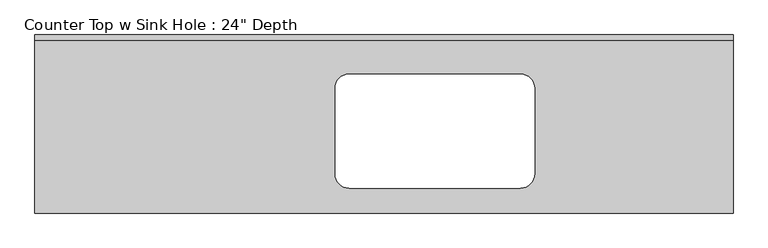
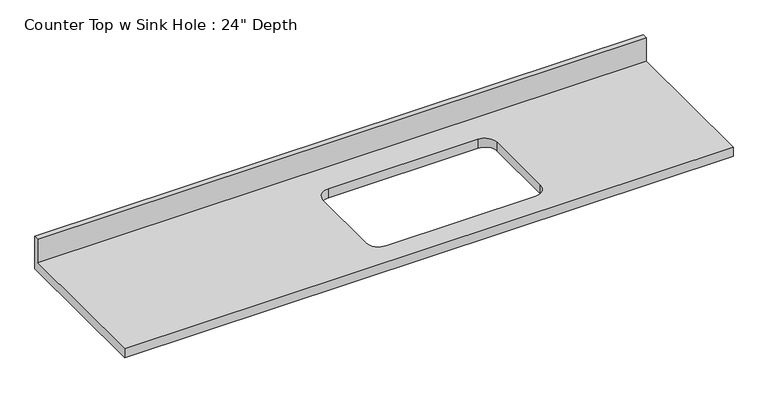
"""IFC4 building model written with IfcOpenShell, lengths in millimetres: furniture geometry."""

from ifc_helpers import new_model, si_unit, frame, origin, place, context, project, spatial, polyline, circle_curve, source, transform, mapped, element, save
from ifc_brep_helpers import plane_surface, revolved_surface, advanced_brep


def furniture_3d2ef6d7(model_context):
    return source(origin(), model_context, "Body", "AdvancedBrep", [
        advanced_brep(
        [(-1200.4622951, -635.0, 914.4), (1288.7377049, -635.0, 914.4), (1288.7377049, -19.05, 914.4), (-1200.4622951, -19.05, 914.4), (-79.6872951, -139.7, 914.4), (529.9127049, -139.7, 914.4), (580.7127049, -190.5, 914.4), (580.7127049, -495.3, 914.4), (529.9127049, -546.1, 914.4), (-79.6872951, -546.1, 914.4), (-130.4872951, -495.3, 914.4), (-130.4872951, -190.5, 914.4), (1288.7377049, 0.0, 876.3), (1288.7377049, -635.0, 876.3), (-1200.4622951, -635.0, 876.3), (-1200.4622951, 0.0, 876.3), (529.9127049, -139.7, 876.3), (-79.6872951, -139.7, 876.3), (-130.4872951, -190.5, 876.3), (-130.4872951, -495.3, 876.3), (-79.6872951, -546.1, 876.3), (529.9127049, -546.1, 876.3), (580.7127049, -495.3, 876.3), (580.7127049, -190.5, 876.3), (-1200.4622951, 0.0, 1016.0), (1288.7377049, 0.0, 1016.0), (-1200.4622951, -19.05, 1016.0), (1288.7377049, -19.05, 1016.0)],
        [
            (0, 1),
            (1, 2),
            (2, 3),
            (3, 0),
            (4, 5),
            (5, 6, circle_curve(frame((529.9127049, -190.5, 914.4), z_axis=(0.0, 0.0, -1.0), x_axis=(1.0, 0.0, 0.0)), 50.8)),
            (6, 7),
            (7, 8, circle_curve(frame((529.9127049, -495.3, 914.4), z_axis=(0.0, 0.0, -1.0), x_axis=(1.0, 0.0, 0.0)), 50.8)),
            (8, 9),
            (9, 10, circle_curve(frame((-79.6872951, -495.3, 914.4), z_axis=(0.0, 0.0, -1.0), x_axis=(1.0, 0.0, 0.0)), 50.8)),
            (10, 11),
            (11, 4, circle_curve(frame((-79.6872951, -190.5, 914.4), z_axis=(0.0, 0.0, -1.0), x_axis=(1.0, 0.0, 0.0)), 50.8)),
            (12, 13),
            (13, 14),
            (14, 15),
            (15, 12),
            (16, 17),
            (17, 18, circle_curve(frame((-79.6872951, -190.5, 876.3), z_axis=(0.0, 0.0, 1.0), x_axis=(1.0, 0.0, 0.0)), 50.8)),
            (18, 19),
            (19, 20, circle_curve(frame((-79.6872951, -495.3, 876.3), z_axis=(0.0, 0.0, 1.0), x_axis=(1.0, 0.0, 0.0)), 50.8)),
            (20, 21),
            (21, 22, circle_curve(frame((529.9127049, -495.3, 876.3), z_axis=(0.0, 0.0, 1.0), x_axis=(1.0, 0.0, 0.0)), 50.8)),
            (22, 23),
            (23, 16, circle_curve(frame((529.9127049, -190.5, 876.3), z_axis=(0.0, 0.0, 1.0), x_axis=(1.0, 0.0, 0.0)), 50.8)),
            (15, 24),
            (24, 25),
            (25, 12),
            (14, 0),
            (3, 26),
            (26, 24),
            (13, 1),
            (25, 27),
            (27, 2),
            (26, 27),
            (4, 17),
            (16, 5),
            (11, 18),
            (10, 19),
            (9, 20),
            (8, 21),
            (7, 22),
            (6, 23),
        ],
        [
            plane_surface(frame((-1200.4622951, 0.0, 914.4), z_axis=(0.0, 0.0, 1.0), x_axis=(-1.0, 0.0, 0.0))),
            plane_surface(frame((-1200.4622951, 0.0, 876.3), z_axis=(0.0, 0.0, -1.0), x_axis=(1.0, 0.0, 0.0))),
            plane_surface(frame((1288.7377049, 0.0, 914.4), z_axis=(0.0, 1.0, 0.0), x_axis=(0.0, 0.0, -1.0))),
            plane_surface(frame((-1200.4622951, 0.0, 914.4), z_axis=(-1.0, 0.0, 0.0), x_axis=(0.0, 0.0, -1.0))),
            plane_surface(frame((-1200.4622951, -635.0, 914.4), z_axis=(0.0, -1.0, 0.0), x_axis=(0.0, 0.0, -1.0))),
            plane_surface(frame((1288.7377049, -635.0, 914.4), z_axis=(1.0, 0.0, 0.0), x_axis=(0.0, 0.0, -1.0))),
            plane_surface(frame((-1200.4622951, 0.0, 1016.0), z_axis=(0.0, 0.0, 1.0), x_axis=(0.0, -1.0, 0.0))),
            plane_surface(frame((-1200.4622951, -19.05, 1016.0), z_axis=(0.0, -1.0, 0.0), x_axis=(0.0, 0.0, -1.0))),
            plane_surface(frame((529.9127049, -139.7, 914.4), z_axis=(0.0, -1.0, 0.0), x_axis=(0.0, 0.0, -1.0))),
            revolved_surface(polyline([(-28.887295100000003, -190.5, 914.4), (-28.887295100000003, -190.5, 876.3)]), (-79.6872951, -190.5, 876.3), (0.0, 0.0, 1.0)),
            plane_surface(frame((-130.4872951, -190.5, 914.4), z_axis=(1.0, 0.0, 0.0), x_axis=(0.0, 0.0, -1.0))),
            revolved_surface(polyline([(-28.887295100000003, -495.3, 914.4), (-28.887295100000003, -495.3, 876.3)]), (-79.6872951, -495.3, 876.3), (0.0, 0.0, 1.0)),
            plane_surface(frame((-79.6872951, -546.1, 914.4), z_axis=(0.0, 1.0, 0.0), x_axis=(0.0, 0.0, -1.0))),
            revolved_surface(polyline([(580.7127049, -495.3, 914.4), (580.7127049, -495.3, 876.3)]), (529.9127049, -495.3, 876.3), (0.0, 0.0, 1.0)),
            plane_surface(frame((580.7127049, -495.3, 914.4), z_axis=(-1.0, 0.0, 0.0), x_axis=(0.0, 0.0, -1.0))),
            revolved_surface(polyline([(580.7127049, -190.5, 914.4), (580.7127049, -190.5, 876.3)]), (529.9127049, -190.5, 876.3), (0.0, 0.0, 1.0)),
        ],
        [
            (0, [[1, 2, 3, 4], [5, 6, 7, 8, 9, 10, 11, 12]]),
            (1, [[13, 14, 15, 16], [17, 18, 19, 20, 21, 22, 23, 24]]),
            (2, [[-16, 25, 26, 27]]),
            (3, [[-15, 28, -4, 29, 30, -25]]),
            (4, [[-1, -28, -14, 31]]),
            (5, [[-13, -27, 32, 33, -2, -31]]),
            (6, [[-30, 34, -32, -26]]),
            (7, [[-34, -29, -3, -33]]),
            (8, [[35, -17, 36, -5]]),
            (9, [[-35, -12, 37, -18]]),
            (10, [[-37, -11, 38, -19]]),
            (11, [[-38, -10, 39, -20]]),
            (12, [[-39, -9, 40, -21]]),
            (13, [[-40, -8, 41, -22]]),
            (14, [[-41, -7, 42, -23]]),
            (15, [[-36, -24, -42, -6]]),
        ],
    ),
    ])


if __name__ == "__main__":
    model = new_model("IFC4")
    model_context = context("Model", 3, world=origin())
    ifc_project = project(units=[si_unit("LENGTHUNIT", "METRE", prefix="MILLI")], contexts=[model_context])
    site = spatial("IfcSite", under=ifc_project)
    building = spatial("IfcBuilding", under=site)
    placement = place(None, origin())
    furniture_shape = furniture_3d2ef6d7(model_context)
    element("IfcFurniture", 1, ObjectType="Counter Top w Sink Hole : 24\" Depth", at=placement, inside=building, context=model_context, shape_type="MappedRepresentation", body=[
        mapped(furniture_shape, transform((0.0, 0.0, 0.0), x_axis=(1.0, 0.0, 0.0), y_axis=(0.0, 1.0, 0.0), z_axis=(0.0, 0.0, 1.0))),
    ])
    save(model, "model.ifc")

# Revit data of these elements
# Type "Counter Top w Sink Hole : 24\" Depth"
#   Assembly Code = "C1030400"
#   Counter Thickness = 0' - 1 1/2"
#   Depth = 2' - 1"
#   Height = 3' - 0"
#   Length [instance default] = 8' - 0"
#   Sink Location [instance default] = 2' - 0"
#   Sink Location To Wall [instance default] = 0' - 6"
#   Sink Opening Depth [instance default] = 1' - 3"
#   Sink Opening Width [instance default] = 2' - 3"
#   Counter Top Material = none
#   Default Elevation = 0
# Element 1 (IfcFurniture, "Counter Top w Sink Hole : 24\" Depth")
#   Length = 8' - 2"
#   Sink Location = 4' - 8 1/8"
#   Materials on its faces: "Counter Top"
# Materials
#   "Counter Top": class "Wood", colour RGB 226 177 128, transparency 0
